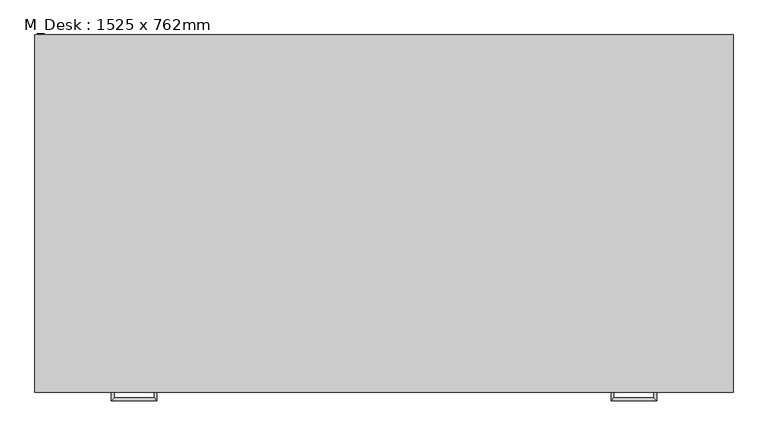
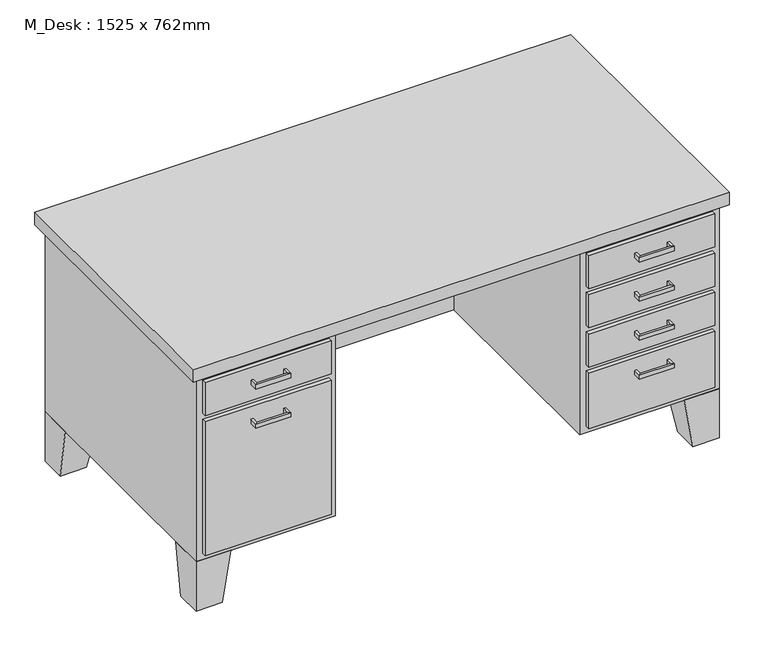
"""IFC4 building model written with IfcOpenShell, lengths in millimetres: furniture geometry, M_Desk : 1525 x 762mm."""

from ifc_helpers import new_model, si_unit, frame, origin, place, context, project, spatial, polyline, outline, extrude, faceted_brep, source, transform, mapped, element, save


def m_desk_1525_x_762mm_8f660baf(model_context):
    return source(origin(), model_context, "Body", "SolidModel", [
        extrude(outline(polyline([(18.55, 0.0), (386.85, 0.0), (386.85, -12.7), (18.55, -12.7), (18.55, 0.0)])), frame((0.0, 0.0, 603.25), z_axis=(0.0, 0.0, 1.0), x_axis=(1.0, 0.0, 0.0)), (0.0, 0.0, 1.0), 101.6),
        extrude(outline(polyline([(18.55, 0.0), (386.85, 0.0), (386.85, -12.7), (18.55, -12.7), (18.55, 0.0)])), frame((0.0, 0.0, 171.05), z_axis=(0.0, 0.0, 1.0), x_axis=(1.0, 0.0, 0.0)), (0.0, 0.0, 1.0), 413.15),
        extrude(outline(polyline([(1137.15, 0.0), (1505.45, 0.0), (1505.45, -12.7), (1137.15, -12.7), (1137.15, 0.0)])), frame((0.0, 0.0, 602.85), z_axis=(0.0, 0.0, 1.0), x_axis=(1.0, 0.0, 0.0)), (0.0, 0.0, 1.0), 102.0),
        extrude(outline(polyline([(1137.15, 0.0), (1505.45, 0.0), (1505.45, -12.7), (1137.15, -12.7), (1137.15, 0.0)])), frame((0.0, 0.0, 171.05), z_axis=(0.0, 0.0, 1.0), x_axis=(1.0, 0.0, 0.0)), (0.0, 0.0, 1.0), 171.45),
        extrude(outline(polyline([(1137.15, 0.0), (1505.45, 0.0), (1505.45, -12.7), (1137.15, -12.7), (1137.15, 0.0)])), frame((0.0, 0.0, 482.2), z_axis=(0.0, 0.0, 1.0), x_axis=(1.0, 0.0, 0.0)), (0.0, 0.0, 1.0), 101.6),
        extrude(outline(polyline([(1137.15, 0.0), (1505.45, 0.0), (1505.45, -12.7), (1137.15, -12.7), (1137.15, 0.0)])), frame((0.0, 0.0, 361.55), z_axis=(0.0, 0.0, 1.0), x_axis=(1.0, 0.0, 0.0)), (0.0, 0.0, 1.0), 101.6),
        faceted_brep([(101.1, 0.0, 152.0), (101.1, 101.6, 152.0), (-0.5, 101.6, 152.0), (-0.5, 0.0, 152.0), (75.7, 0.0, 0.0), (-0.5, 0.0, 0.0), (-0.5, 76.2, 0.0), (75.7, 76.2, 0.0)], [[[0, 1, 2, 3]], [[4, 5, 6, 7]], [[4, 7, 1, 0]], [[7, 6, 2, 1]], [[6, 5, 3, 2]], [[5, 4, 0, 3]]]),
        faceted_brep([(101.1, 762.0, 152.0), (-0.5, 762.0, 152.0), (-0.5, 660.4, 152.0), (101.1, 660.4, 152.0), (75.7, 762.0, 0.0), (75.7, 685.8, 0.0), (-0.5, 685.8, 0.0), (-0.5, 762.0, 0.0)], [[[0, 1, 2, 3]], [[4, 5, 6, 7]], [[4, 7, 1, 0]], [[7, 6, 2, 1]], [[6, 5, 3, 2]], [[5, 4, 0, 3]]]),
        faceted_brep([(1422.9, 762.0, 152.0), (1422.9, 660.4, 152.0), (1524.5, 660.4, 152.0), (1524.5, 762.0, 152.0), (1448.3, 762.0, 0.0), (1524.5, 762.0, 0.0), (1524.5, 685.8, 0.0), (1448.3, 685.8, 0.0)], [[[0, 1, 2, 3]], [[4, 5, 6, 7]], [[4, 7, 1, 0]], [[7, 6, 2, 1]], [[6, 5, 3, 2]], [[5, 4, 0, 3]]]),
        faceted_brep([(1422.9, 0.0, 152.0), (1524.5, 0.0, 152.0), (1524.5, 101.6, 152.0), (1422.9, 101.6, 152.0), (1448.3, 0.0, 0.0), (1448.3, 76.2, 0.0), (1524.5, 76.2, 0.0), (1524.5, 0.0, 0.0)], [[[0, 1, 2, 3]], [[4, 5, 6, 7]], [[4, 7, 1, 0]], [[7, 6, 2, 1]], [[6, 5, 3, 2]], [[5, 4, 0, 3]]]),
        extrude(outline(polyline([(-19.55, -19.05), (-19.55, 781.05), (1543.55, 781.05), (1543.55, -19.05), (-19.55, -19.05)])), frame((0.0, 0.0, 723.9), z_axis=(0.0, 0.0, 1.0), x_axis=(1.0, 0.0, 0.0)), (0.0, 0.0, 1.0), 38.1),
        extrude(outline(polyline([(1118.1, 0.0), (1118.1, 635.0), (405.9, 635.0), (405.9, 0.0), (-0.5, 0.0), (-0.5, 762.0), (1524.5, 762.0), (1524.5, 0.0), (1118.1, 0.0)])), frame((0.0, 0.0, 152.0), z_axis=(0.0, 0.0, 1.0), x_axis=(1.0, 0.0, 0.0)), (0.0, 0.0, 1.0), 571.9),
        faceted_brep([(158.25, -12.7, 546.1), (158.25, -12.7, 533.4), (151.9, -12.7, 533.4), (151.9, -12.7, 546.1), (158.25, -31.75, 546.1), (158.25, -31.75, 533.4), (151.9, -38.1, 533.4), (151.9, -38.1, 546.1), (247.15, -31.75, 546.1), (247.15, -31.75, 533.4), (253.5, -38.1, 533.4), (253.5, -38.1, 546.1), (247.15, -12.7, 546.1), (253.5, -12.7, 546.1), (253.5, -12.7, 533.4), (247.15, -12.7, 533.4)], [[[0, 1, 2, 3]], [[1, 0, 4, 5]], [[2, 1, 5, 6]], [[3, 2, 6, 7]], [[0, 3, 7, 4]], [[5, 4, 8, 9]], [[6, 5, 9, 10]], [[7, 6, 10, 11]], [[4, 7, 11, 8]], [[12, 13, 14, 15]], [[9, 8, 12, 15]], [[10, 9, 15, 14]], [[11, 10, 14, 13]], [[8, 11, 13, 12]]]),
        faceted_brep([(158.25, -12.7, 666.75), (158.25, -12.7, 654.05), (151.9, -12.7, 654.05), (151.9, -12.7, 666.75), (158.25, -31.75, 666.75), (158.25, -31.75, 654.05), (151.9, -38.1, 654.05), (151.9, -38.1, 666.75), (247.15, -31.75, 666.75), (247.15, -31.75, 654.05), (253.5, -38.1, 654.05), (253.5, -38.1, 666.75), (247.15, -12.7, 666.75), (253.5, -12.7, 666.75), (253.5, -12.7, 654.05), (247.15, -12.7, 654.05)], [[[0, 1, 2, 3]], [[1, 0, 4, 5]], [[2, 1, 5, 6]], [[3, 2, 6, 7]], [[0, 3, 7, 4]], [[5, 4, 8, 9]], [[6, 5, 9, 10]], [[7, 6, 10, 11]], [[4, 7, 11, 8]], [[12, 13, 14, 15]], [[9, 8, 12, 15]], [[10, 9, 15, 14]], [[11, 10, 14, 13]], [[8, 11, 13, 12]]]),
        faceted_brep([(1365.75, -12.7, 304.8), (1372.1, -12.7, 304.8), (1372.1, -12.7, 292.1), (1365.75, -12.7, 292.1), (1365.75, -31.75, 304.8), (1372.1, -38.1, 304.8), (1372.1, -38.1, 292.1), (1365.75, -31.75, 292.1), (1276.85, -31.75, 304.8), (1270.5, -38.1, 304.8), (1270.5, -38.1, 292.1), (1276.85, -31.75, 292.1), (1276.85, -12.7, 304.8), (1276.85, -12.7, 292.1), (1270.5, -12.7, 292.1), (1270.5, -12.7, 304.8)], [[[0, 1, 2, 3]], [[1, 0, 4, 5]], [[2, 1, 5, 6]], [[3, 2, 6, 7]], [[0, 3, 7, 4]], [[5, 4, 8, 9]], [[6, 5, 9, 10]], [[7, 6, 10, 11]], [[4, 7, 11, 8]], [[12, 13, 14, 15]], [[9, 8, 12, 15]], [[10, 9, 15, 14]], [[11, 10, 14, 13]], [[8, 11, 13, 12]]]),
        faceted_brep([(1365.75, -12.7, 425.45), (1372.1, -12.7, 425.45), (1372.1, -12.7, 412.75), (1365.75, -12.7, 412.75), (1365.75, -31.75, 425.45), (1372.1, -38.1, 425.45), (1372.1, -38.1, 412.75), (1365.75, -31.75, 412.75), (1276.85, -31.75, 425.45), (1270.5, -38.1, 425.45), (1270.5, -38.1, 412.75), (1276.85, -31.75, 412.75), (1276.85, -12.7, 425.45), (1276.85, -12.7, 412.75), (1270.5, -12.7, 412.75), (1270.5, -12.7, 425.45)], [[[0, 1, 2, 3]], [[1, 0, 4, 5]], [[2, 1, 5, 6]], [[3, 2, 6, 7]], [[0, 3, 7, 4]], [[5, 4, 8, 9]], [[6, 5, 9, 10]], [[7, 6, 10, 11]], [[4, 7, 11, 8]], [[12, 13, 14, 15]], [[9, 8, 12, 15]], [[10, 9, 15, 14]], [[11, 10, 14, 13]], [[8, 11, 13, 12]]]),
        faceted_brep([(1365.75, -12.7, 546.1), (1372.1, -12.7, 546.1), (1372.1, -12.7, 533.4), (1365.75, -12.7, 533.4), (1365.75, -31.75, 546.1), (1372.1, -38.1, 546.1), (1372.1, -38.1, 533.4), (1365.75, -31.75, 533.4), (1276.85, -31.75, 546.1), (1270.5, -38.1, 546.1), (1270.5, -38.1, 533.4), (1276.85, -31.75, 533.4), (1276.85, -12.7, 546.1), (1276.85, -12.7, 533.4), (1270.5, -12.7, 533.4), (1270.5, -12.7, 546.1)], [[[0, 1, 2, 3]], [[1, 0, 4, 5]], [[2, 1, 5, 6]], [[3, 2, 6, 7]], [[0, 3, 7, 4]], [[5, 4, 8, 9]], [[6, 5, 9, 10]], [[7, 6, 10, 11]], [[4, 7, 11, 8]], [[12, 13, 14, 15]], [[9, 8, 12, 15]], [[10, 9, 15, 14]], [[11, 10, 14, 13]], [[8, 11, 13, 12]]]),
        faceted_brep([(1365.75, -12.7, 666.75), (1372.1, -12.7, 666.75), (1372.1, -12.7, 654.05), (1365.75, -12.7, 654.05), (1365.75, -31.75, 666.75), (1372.1, -38.1, 666.75), (1372.1, -38.1, 654.05), (1365.75, -31.75, 654.05), (1276.85, -31.75, 666.75), (1270.5, -38.1, 666.75), (1270.5, -38.1, 654.05), (1276.85, -31.75, 654.05), (1276.85, -12.7, 666.75), (1276.85, -12.7, 654.05), (1270.5, -12.7, 654.05), (1270.5, -12.7, 666.75)], [[[0, 1, 2, 3]], [[1, 0, 4, 5]], [[2, 1, 5, 6]], [[3, 2, 6, 7]], [[0, 3, 7, 4]], [[5, 4, 8, 9]], [[6, 5, 9, 10]], [[7, 6, 10, 11]], [[4, 7, 11, 8]], [[12, 13, 14, 15]], [[9, 8, 12, 15]], [[10, 9, 15, 14]], [[11, 10, 14, 13]], [[8, 11, 13, 12]]]),
    ])


if __name__ == "__main__":
    model = new_model("IFC4")
    model_context = context("Model", 3, world=origin())
    ifc_project = project(units=[si_unit("LENGTHUNIT", "METRE", prefix="MILLI")], contexts=[model_context])
    site = spatial("IfcSite", under=ifc_project)
    building = spatial("IfcBuilding", under=site)
    placement = place(None, origin())
    m_desk_1525_x_762mm_shape = m_desk_1525_x_762mm_8f660baf(model_context)
    element("IfcFurniture", 1, ObjectType="M_Desk : 1525 x 762mm", at=placement, inside=building, context=model_context, shape_type="MappedRepresentation", body=[
        mapped(m_desk_1525_x_762mm_shape, transform((0.0, 0.0, 0.0), x_axis=(1.0, 0.0, 0.0), y_axis=(0.0, 1.0, 0.0), z_axis=(0.0, 0.0, 1.0))),
    ])
    save(model, "model.ifc")

# Revit data of these elements
# Type "M_Desk : 1525 x 762mm"
#   Depth = 762 mm
#   Height = 762 mm
#   Leg Height = 152 mm
#   Width = 1525 mm
#   Body Material = Laminate, Ivory, Matte
#   Handle/Leg Material = Steel, Chrome Plated
#   Top Material = Cherry
#   Default Elevation = 0
#   Assembly Code = ""
# Element 1 (IfcFurniture, "M_Desk : 1525 x 762mm")
#   Materials on its faces: "Steel, Chrome Plated", "Laminate, Ivory, Matte", "Cherry"
# Materials
#   "Laminate, Ivory, Matte": class "Plastic", colour RGB 247 247 229, transparency 0, Description = "Plastic Laminate - Ivory, Matte", Cost = 0
#   "Steel, Chrome Plated": class "Metal", colour RGB 244 244 244, transparency 0, Description = "Chromiuim plated steel", Cost = 0
#   "Cherry": class "Wood", colour RGB 154 107 61, transparency 0, Description = "Prunus Serotina", Cost = 0
